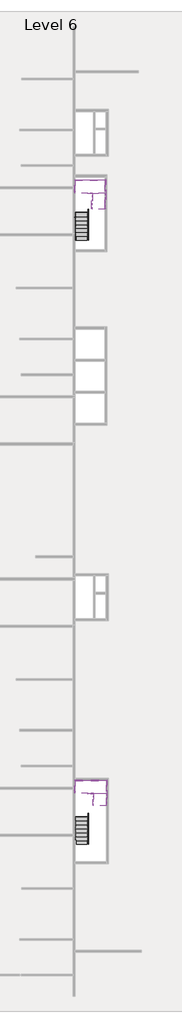
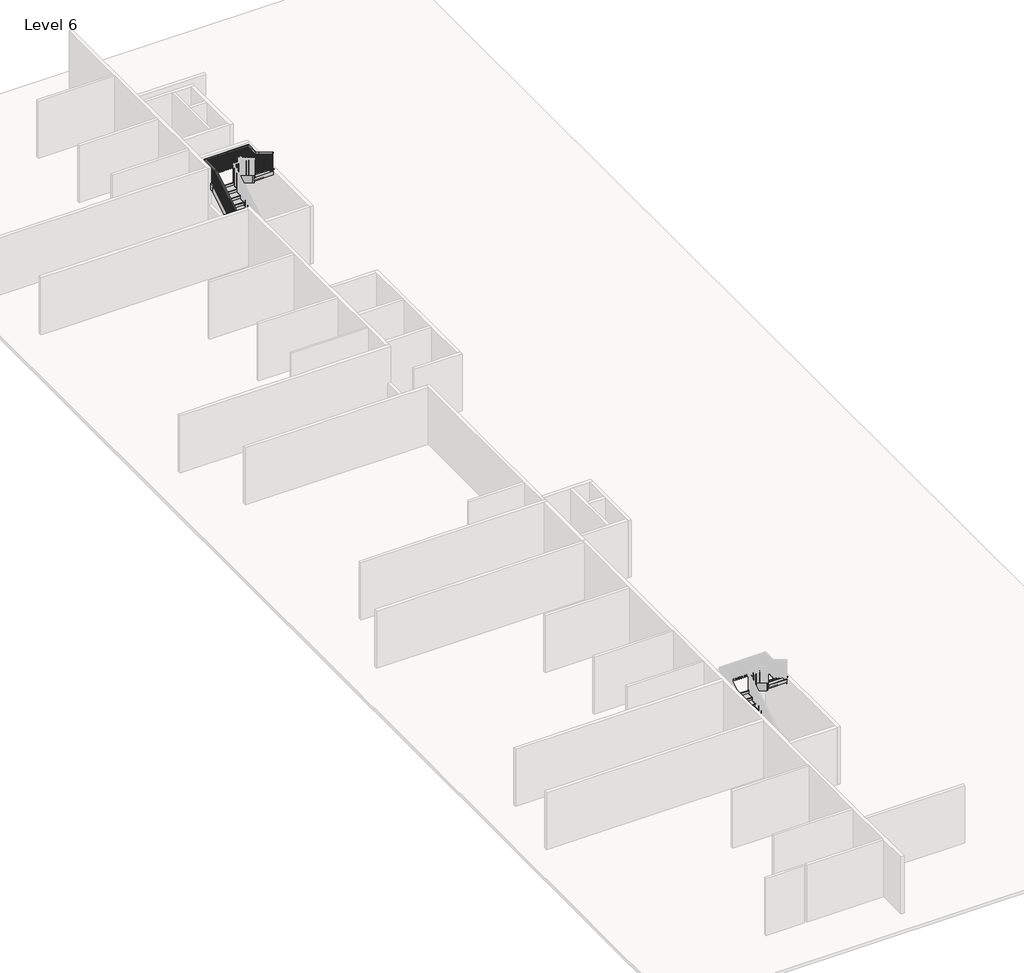
# One storey, part 8 of 8: 16 members, 4 stair flights, 2 slabs, 1 railing.
"""IFC4 building model written with IfcOpenShell, lengths in millimetres."""

from ifc_helpers import new_model, si_unit, frame, origin, place, context, project, spatial, polyline, outline, extrude, faceted_brep, transform, mapped, element, save
from components import non_monolithic_landing_f4425cc3, non_monolithic_landing_d932be8a, stair_flight_a1121a25, stair_flight_592be736, stair_flight_ee9ddb45, stair_flight_fe606327

model = new_model("IFC4")

# Units and contexts
model_context = context("Model", 3, world=origin())
ifc_project = project(units=[si_unit("LENGTHUNIT", "METRE", prefix="MILLI")], contexts=[model_context])

# Site, building, storey
site = spatial("IfcSite", under=ifc_project)
building = spatial("IfcBuilding", under=site)
storey = spatial("IfcBuildingStorey", under=building, Name="Level 6", Elevation=40474.6172466)

# Members
placement = place(None, origin())
element("IfcMember", 1, ObjectType="Stringer - 2\" Width", at=placement, inside=storey, context=model_context, shape_type="SweptSolid", body=[
    extrude(outline(polyline([(-23154.3851539, 40474.6172466), (-23154.3851539, 40686.7317586), (-19467.0440987, 42921.4839133), (-19381.8896422, 42616.6839133), (-22916.2996422, 40474.6172466), (-23154.3851539, 40474.6172466)])), frame((-3668.2415084, 0.0, 0.0), z_axis=(1.0, 0.0, 0.0), x_axis=(0.0, 1.0, 0.0)), (0.0, 0.0, 1.0), 50.8),
])
element("IfcMember", 2, ObjectType="Stringer - 2\" Width", at=placement, inside=storey, context=model_context, shape_type="SweptSolid", body=[
    extrude(outline(polyline([(-23154.3851539, 40474.6172466), (-23154.3851539, 40686.7317586), (-19572.9851539, 42857.2772131), (-19572.9851539, 42500.8684516), (-22916.2996422, 40474.6172466), (-23154.3851539, 40474.6172466)])), frame((-2703.0415084, 0.0, 0.0), z_axis=(1.0, 0.0, 0.0), x_axis=(0.0, 1.0, 0.0)), (0.0, 0.0, 1.0), 50.8),
])
element("IfcMember", 3, ObjectType="Stringer - 2\" Width", at=placement, inside=storey, context=model_context, shape_type="SweptSolid", body=[
    extrude(outline(polyline([(-19297.9262092, 42921.4839133), (-19383.0806657, 42616.6839133), (-20360.3851539, 43208.9896637), (-20360.3851539, 43565.3984252), (-19297.9262092, 42921.4839133)])), frame((-1382.2415084, 0.0, 0.0), z_axis=(1.0, 0.0, 0.0), x_axis=(0.0, 1.0, 0.0)), (0.0, 0.0, 1.0), 50.8),
])
element("IfcMember", 4, ObjectType="Stringer - 2\" Width", at=placement, inside=storey, context=model_context, shape_type="SweptSolid", body=[
    extrude(outline(polyline([(-19522.1851539, 43057.3984252), (-19522.1851539, 42700.9896637), (-20360.3851539, 43208.9896637), (-20360.3851539, 43565.3984252), (-19522.1851539, 43057.3984252)])), frame((-2347.4415084, 0.0, 0.0), z_axis=(1.0, 0.0, 0.0), x_axis=(0.0, 1.0, 0.0)), (0.0, 0.0, 1.0), 50.8),
])
element("IfcMember", 5, ObjectType="Stringer - 2\" Width", at=placement, inside=storey, context=model_context, shape_type="Brep", body=[
    faceted_brep([(-1382.2415084, -19297.9262092, 42921.4839133), (-1331.4415084, -19297.9262092, 42921.4839133), (-1331.4415084, -18556.9851539, 42921.4839133), (-1382.2415084, -18607.7851539, 42921.4839133), (-1382.2415084, -19383.0806657, 42616.6839133), (-1382.2415084, -18607.7851539, 42616.6839133), (-1331.4415084, -19383.0806657, 42616.6839133), (-1331.4415084, -18556.9851539, 42616.6839133)], [[[0, 1, 2, 3]], [[4, 0, 3, 5]], [[6, 4, 5, 7]], [[1, 6, 7, 2]], [[1, 0, 4, 6]], [[2, 7, 5, 3]]]),
])
element("IfcMember", 6, ObjectType="Stringer - 2\" Width", at=placement, inside=storey, context=model_context, shape_type="SweptSolid", body=[
    extrude(outline(polyline([(-1331.4415084, -18556.9851539), (-1382.2415084, -18607.7851539), (-3617.4415084, -18607.7851539), (-3668.2415084, -18556.9851539), (-1331.4415084, -18556.9851539)])), frame((0.0, 0.0, 42616.6839133), z_axis=(0.0, 0.0, 1.0), x_axis=(1.0, 0.0, 0.0)), (0.0, 0.0, 1.0), 304.8),
])
element("IfcMember", 7, ObjectType="Stringer - 2\" Width", at=placement, inside=storey, context=model_context, shape_type="Brep", body=[
    faceted_brep([(-3617.4415084, -18607.7851539, 42921.4839133), (-3668.2415084, -18556.9851539, 42921.4839133), (-3668.2415084, -19467.0440987, 42921.4839133), (-3617.4415084, -19467.0440987, 42921.4839133), (-3617.4415084, -18607.7851539, 42616.6839133), (-3617.4415084, -19381.8896422, 42616.6839133), (-3668.2415084, -18556.9851539, 42616.6839133), (-3668.2415084, -19381.8896422, 42616.6839133)], [[[0, 1, 2, 3]], [[4, 0, 3, 5]], [[6, 4, 5, 7]], [[1, 6, 7, 2]], [[1, 0, 4, 6]], [[2, 7, 5, 3]]]),
])
element("IfcMember", 8, ObjectType="Stringer - 2\" Width", at=placement, inside=storey, context=model_context, shape_type="SweptSolid", body=[
    extrude(outline(polyline([(-2703.0415084, -19572.9851539), (-2703.0415084, -19522.1851539), (-2347.4415084, -19522.1851539), (-2347.4415084, -19572.9851539), (-2703.0415084, -19572.9851539)])), frame((0.0, 0.0, 42616.6839133), z_axis=(0.0, 0.0, 1.0), x_axis=(1.0, 0.0, 0.0)), (0.0, 0.0, 1.0), 304.8),
])
element("IfcMember", 9, ObjectType="Stringer - 2\" Width", at=placement, inside=storey, context=model_context, shape_type="SweptSolid", body=[
    extrude(outline(polyline([(19841.9216096, 40474.6172466), (19841.9216096, 40686.7317586), (23249.8626649, 42752.1505799), (23335.0171214, 42447.3505799), (20080.0071214, 40474.6172466), (19841.9216096, 40474.6172466)])), frame((-3668.2415084, 0.0, 0.0), z_axis=(1.0, 0.0, 0.0), x_axis=(0.0, 1.0, 0.0)), (0.0, 0.0, 1.0), 50.8),
])
element("IfcMember", 10, ObjectType="Stringer - 2\" Width", at=placement, inside=storey, context=model_context, shape_type="SweptSolid", body=[
    extrude(outline(polyline([(19841.9216096, 40474.6172466), (19841.9216096, 40686.7317586), (23143.9216096, 42687.9438798), (23143.9216096, 42331.5351183), (20080.0071214, 40474.6172466), (19841.9216096, 40474.6172466)])), frame((-2703.0415084, 0.0, 0.0), z_axis=(1.0, 0.0, 0.0), x_axis=(0.0, 1.0, 0.0)), (0.0, 0.0, 1.0), 50.8),
])
element("IfcMember", 11, ObjectType="Stringer - 2\" Width", at=placement, inside=storey, context=model_context, shape_type="SweptSolid", body=[
    extrude(outline(polyline([(23418.9805543, 42752.1505799), (23333.8260978, 42447.3505799), (22077.1216096, 43208.9896637), (22077.1216096, 43565.3984252), (23418.9805543, 42752.1505799)])), frame((-1483.8415084, 0.0, 0.0), z_axis=(1.0, 0.0, 0.0), x_axis=(0.0, 1.0, 0.0)), (0.0, 0.0, 1.0), 50.8),
])
element("IfcMember", 12, ObjectType="Stringer - 2\" Width", at=placement, inside=storey, context=model_context, shape_type="SweptSolid", body=[
    extrude(outline(polyline([(23194.7216096, 42888.0650919), (23194.7216096, 42531.6563304), (22077.1216096, 43208.9896637), (22077.1216096, 43565.3984252), (23194.7216096, 42888.0650919)])), frame((-2449.0415084, 0.0, 0.0), z_axis=(1.0, 0.0, 0.0), x_axis=(0.0, 1.0, 0.0)), (0.0, 0.0, 1.0), 50.8),
])
element("IfcMember", 13, ObjectType="Stringer - 2\" Width", at=placement, inside=storey, context=model_context, shape_type="Brep", body=[
    faceted_brep([(-1483.8415084, 23418.9805543, 42752.1505799), (-1433.0415084, 23418.9805543, 42752.1505799), (-1433.0415084, 24159.9216096, 42752.1505799), (-1483.8415084, 24109.1216096, 42752.1505799), (-1483.8415084, 23333.8260978, 42447.3505799), (-1483.8415084, 24109.1216096, 42447.3505799), (-1433.0415084, 23333.8260978, 42447.3505799), (-1433.0415084, 24159.9216096, 42447.3505799)], [[[0, 1, 2, 3]], [[4, 0, 3, 5]], [[6, 4, 5, 7]], [[1, 6, 7, 2]], [[1, 0, 4, 6]], [[2, 7, 5, 3]]]),
])
element("IfcMember", 14, ObjectType="Stringer - 2\" Width", at=placement, inside=storey, context=model_context, shape_type="SweptSolid", body=[
    extrude(outline(polyline([(-1433.0415084, 24159.9216096), (-1483.8415084, 24109.1216096), (-3617.4415084, 24109.1216096), (-3668.2415084, 24159.9216096), (-1433.0415084, 24159.9216096)])), frame((0.0, 0.0, 42447.3505799), z_axis=(0.0, 0.0, 1.0), x_axis=(1.0, 0.0, 0.0)), (0.0, 0.0, 1.0), 304.8),
])
element("IfcMember", 15, ObjectType="Stringer - 2\" Width", at=placement, inside=storey, context=model_context, shape_type="Brep", body=[
    faceted_brep([(-3617.4415084, 24109.1216096, 42752.1505799), (-3668.2415084, 24159.9216096, 42752.1505799), (-3668.2415084, 23249.8626649, 42752.1505799), (-3617.4415084, 23249.8626649, 42752.1505799), (-3617.4415084, 24109.1216096, 42447.3505799), (-3617.4415084, 23335.0171214, 42447.3505799), (-3668.2415084, 24159.9216096, 42447.3505799), (-3668.2415084, 23335.0171214, 42447.3505799)], [[[0, 1, 2, 3]], [[4, 0, 3, 5]], [[6, 4, 5, 7]], [[1, 6, 7, 2]], [[1, 0, 4, 6]], [[2, 7, 5, 3]]]),
])
element("IfcMember", 16, ObjectType="Stringer - 2\" Width", at=placement, inside=storey, context=model_context, shape_type="SweptSolid", body=[
    extrude(outline(polyline([(-2703.0415084, 23143.9216096), (-2703.0415084, 23194.7216096), (-2449.0415084, 23194.7216096), (-2449.0415084, 23143.9216096), (-2703.0415084, 23143.9216096)])), frame((0.0, 0.0, 42447.3505799), z_axis=(0.0, 0.0, 1.0), x_axis=(1.0, 0.0, 0.0)), (0.0, 0.0, 1.0), 304.8),
])

# Railing
element("IfcRailing", 17, ObjectType="Handrail - Rectangular", at=placement, inside=storey, context=model_context, shape_type="SolidModel", body=[
    faceted_brep([(-3617.4415084, 19841.9216096, 41558.3505799), (-3617.4415084, 19841.9216096, 41498.9491197), (-3566.6415084, 19841.9216096, 41498.9491197), (-3566.6415084, 19841.9216096, 41558.3505799), (-3617.4415084, 23194.7216096, 43590.3505799), (-3617.4415084, 23208.914019, 43539.5505799), (-3566.6415084, 23208.914019, 43539.5505799), (-3566.6415084, 23194.7216096, 43590.3505799), (-3617.4415084, 24109.1216096, 43590.3505799), (-3617.4415084, 24109.1216096, 43539.5505799), (-3566.6415084, 24058.3216096, 43539.5505799), (-3566.6415084, 24058.3216096, 43590.3505799), (-1483.8415084, 24109.1216096, 43590.3505799), (-1483.8415084, 24109.1216096, 43539.5505799), (-1534.6415084, 24058.3216096, 43539.5505799), (-1534.6415084, 24058.3216096, 43590.3505799), (-1483.8415084, 23474.1216096, 43590.3505799), (-1483.8415084, 23459.9292002, 43539.5505799), (-1534.6415084, 23459.9292002, 43539.5505799), (-1534.6415084, 23474.1216096, 43590.3505799), (-1483.8415084, 23194.7216096, 43759.6839133), (-1483.8415084, 23168.3918824, 43716.2398634), (-1534.6415084, 23168.3918824, 43716.2398634), (-1534.6415084, 23194.7216096, 43759.6839133), (-1483.8415084, 22077.1216096, 44437.0172466), (-1534.6415084, 22077.1216096, 44437.0172466), (-1534.6415084, 22077.1216096, 44377.6157863), (-1483.8415084, 22077.1216096, 44377.6157863)], [[[0, 1, 2, 3]], [[1, 0, 4, 5]], [[2, 1, 5, 6]], [[3, 2, 6, 7]], [[0, 3, 7, 4]], [[5, 4, 8, 9]], [[6, 5, 9, 10]], [[7, 6, 10, 11]], [[4, 7, 11, 8]], [[9, 8, 12, 13]], [[10, 9, 13, 14]], [[11, 10, 14, 15]], [[8, 11, 15, 12]], [[13, 12, 16, 17]], [[14, 13, 17, 18]], [[15, 14, 18, 19]], [[12, 15, 19, 16]], [[17, 16, 20, 21]], [[18, 17, 21, 22]], [[19, 18, 22, 23]], [[16, 19, 23, 20]], [[24, 25, 26, 27]], [[21, 20, 24, 27]], [[22, 21, 27, 26]], [[23, 22, 26, 25]], [[20, 23, 25, 24]]]),
    extrude(outline(polyline([(22188.2466096, 44310.2673015), (22188.2466096, 43353.2839133), (22169.1966096, 43353.2839133), (22169.1966096, 44321.812756), (22188.2466096, 44310.2673015)])), frame((-1518.7665084, 0.0, 0.0), z_axis=(1.0, 0.0, 0.0), x_axis=(0.0, 1.0, 0.0)), (0.0, 0.0, 1.0), 19.05),
    extrude(outline(polyline([(22289.8466096, 44248.6915439), (22289.8466096, 43353.2839133), (22270.7966096, 43353.2839133), (22270.7966096, 44260.2369985), (22289.8466096, 44248.6915439)])), frame((-1518.7665084, 0.0, 0.0), z_axis=(1.0, 0.0, 0.0), x_axis=(0.0, 1.0, 0.0)), (0.0, 0.0, 1.0), 19.05),
    extrude(outline(polyline([(22391.4466096, 44187.1157863), (22391.4466096, 43183.9505799), (22372.3966096, 43183.9505799), (22372.3966096, 44198.6612409), (22391.4466096, 44187.1157863)])), frame((-1518.7665084, 0.0, 0.0), z_axis=(1.0, 0.0, 0.0), x_axis=(0.0, 1.0, 0.0)), (0.0, 0.0, 1.0), 19.05),
    extrude(outline(polyline([(22493.0466096, 44125.5400288), (22493.0466096, 43183.9505799), (22473.9966096, 43183.9505799), (22473.9966096, 44137.0854833), (22493.0466096, 44125.5400288)])), frame((-1518.7665084, 0.0, 0.0), z_axis=(1.0, 0.0, 0.0), x_axis=(0.0, 1.0, 0.0)), (0.0, 0.0, 1.0), 19.05),
    extrude(outline(polyline([(22594.6466096, 44063.9642712), (22594.6466096, 43183.9505799), (22575.5966096, 43183.9505799), (22575.5966096, 44075.5097257), (22594.6466096, 44063.9642712)])), frame((-1518.7665084, 0.0, 0.0), z_axis=(1.0, 0.0, 0.0), x_axis=(0.0, 1.0, 0.0)), (0.0, 0.0, 1.0), 19.05),
    extrude(outline(polyline([(22696.2466096, 44002.3885136), (22696.2466096, 43014.6172466), (22677.1966096, 43014.6172466), (22677.1966096, 44013.9339682), (22696.2466096, 44002.3885136)])), frame((-1518.7665084, 0.0, 0.0), z_axis=(1.0, 0.0, 0.0), x_axis=(0.0, 1.0, 0.0)), (0.0, 0.0, 1.0), 19.05),
    extrude(outline(polyline([(22797.8466096, 43940.812756), (22797.8466096, 43014.6172466), (22778.7966096, 43014.6172466), (22778.7966096, 43952.3582106), (22797.8466096, 43940.812756)])), frame((-1518.7665084, 0.0, 0.0), z_axis=(1.0, 0.0, 0.0), x_axis=(0.0, 1.0, 0.0)), (0.0, 0.0, 1.0), 19.05),
    extrude(outline(polyline([(22899.4466096, 43879.2369985), (22899.4466096, 43014.6172466), (22880.3966096, 43014.6172466), (22880.3966096, 43890.782453), (22899.4466096, 43879.2369985)])), frame((-1518.7665084, 0.0, 0.0), z_axis=(1.0, 0.0, 0.0), x_axis=(0.0, 1.0, 0.0)), (0.0, 0.0, 1.0), 19.05),
    extrude(outline(polyline([(23001.0466096, 43817.6612409), (23001.0466096, 42845.2839133), (22981.9966096, 42845.2839133), (22981.9966096, 43829.2066954), (23001.0466096, 43817.6612409)])), frame((-1518.7665084, 0.0, 0.0), z_axis=(1.0, 0.0, 0.0), x_axis=(0.0, 1.0, 0.0)), (0.0, 0.0, 1.0), 19.05),
    extrude(outline(polyline([(23102.6466096, 43756.0854833), (23102.6466096, 42845.2839133), (23083.5966096, 42845.2839133), (23083.5966096, 43767.6309379), (23102.6466096, 43756.0854833)])), frame((-1518.7665084, 0.0, 0.0), z_axis=(1.0, 0.0, 0.0), x_axis=(0.0, 1.0, 0.0)), (0.0, 0.0, 1.0), 19.05),
    extrude(outline(polyline([(23280.4466096, 43648.3279076), (23280.4466096, 42675.9505799), (23261.3966096, 42675.9505799), (23261.3966096, 43659.8733621), (23280.4466096, 43648.3279076)])), frame((-1518.7665084, 0.0, 0.0), z_axis=(1.0, 0.0, 0.0), x_axis=(0.0, 1.0, 0.0)), (0.0, 0.0, 1.0), 19.05),
    extrude(outline(polyline([(23382.0466096, 43586.75215), (23382.0466096, 42675.9505799), (23362.9966096, 42675.9505799), (23362.9966096, 43598.2976045), (23382.0466096, 43586.75215)])), frame((-1518.7665084, 0.0, 0.0), z_axis=(1.0, 0.0, 0.0), x_axis=(0.0, 1.0, 0.0)), (0.0, 0.0, 1.0), 19.05),
    extrude(outline(polyline([(-1499.7165084, 23483.6466096), (-1499.7165084, 23464.5966096), (-1518.7665084, 23464.5966096), (-1518.7665084, 23483.6466096), (-1499.7165084, 23483.6466096)])), frame((0.0, 0.0, 42675.9505799), z_axis=(0.0, 0.0, 1.0), x_axis=(1.0, 0.0, 0.0)), (0.0, 0.0, 1.0), 863.6),
    extrude(outline(polyline([(-1499.7165084, 23585.2466096), (-1499.7165084, 23566.1966096), (-1518.7665084, 23566.1966096), (-1518.7665084, 23585.2466096), (-1499.7165084, 23585.2466096)])), frame((0.0, 0.0, 42675.9505799), z_axis=(0.0, 0.0, 1.0), x_axis=(1.0, 0.0, 0.0)), (0.0, 0.0, 1.0), 863.6),
    extrude(outline(polyline([(-1499.7165084, 23686.8466096), (-1499.7165084, 23667.7966096), (-1518.7665084, 23667.7966096), (-1518.7665084, 23686.8466096), (-1499.7165084, 23686.8466096)])), frame((0.0, 0.0, 42675.9505799), z_axis=(0.0, 0.0, 1.0), x_axis=(1.0, 0.0, 0.0)), (0.0, 0.0, 1.0), 863.6),
    extrude(outline(polyline([(-1499.7165084, 23788.4466096), (-1499.7165084, 23769.3966096), (-1518.7665084, 23769.3966096), (-1518.7665084, 23788.4466096), (-1499.7165084, 23788.4466096)])), frame((0.0, 0.0, 42675.9505799), z_axis=(0.0, 0.0, 1.0), x_axis=(1.0, 0.0, 0.0)), (0.0, 0.0, 1.0), 863.6),
    extrude(outline(polyline([(-1499.7165084, 23890.0466096), (-1499.7165084, 23870.9966096), (-1518.7665084, 23870.9966096), (-1518.7665084, 23890.0466096), (-1499.7165084, 23890.0466096)])), frame((0.0, 0.0, 42675.9505799), z_axis=(0.0, 0.0, 1.0), x_axis=(1.0, 0.0, 0.0)), (0.0, 0.0, 1.0), 863.6),
    extrude(outline(polyline([(-1499.7165084, 23991.6466096), (-1499.7165084, 23972.5966096), (-1518.7665084, 23972.5966096), (-1518.7665084, 23991.6466096), (-1499.7165084, 23991.6466096)])), frame((0.0, 0.0, 42675.9505799), z_axis=(0.0, 0.0, 1.0), x_axis=(1.0, 0.0, 0.0)), (0.0, 0.0, 1.0), 863.6),
    extrude(outline(polyline([(-1569.5665084, 24093.2466096), (-1550.5165084, 24093.2466096), (-1550.5165084, 24074.1966096), (-1569.5665084, 24074.1966096), (-1569.5665084, 24093.2466096)])), frame((0.0, 0.0, 42675.9505799), z_axis=(0.0, 0.0, 1.0), x_axis=(1.0, 0.0, 0.0)), (0.0, 0.0, 1.0), 863.6),
    extrude(outline(polyline([(-1671.1665084, 24093.2466096), (-1652.1165084, 24093.2466096), (-1652.1165084, 24074.1966096), (-1671.1665084, 24074.1966096), (-1671.1665084, 24093.2466096)])), frame((0.0, 0.0, 42675.9505799), z_axis=(0.0, 0.0, 1.0), x_axis=(1.0, 0.0, 0.0)), (0.0, 0.0, 1.0), 863.6),
    extrude(outline(polyline([(-1772.7665084, 24093.2466096), (-1753.7165084, 24093.2466096), (-1753.7165084, 24074.1966096), (-1772.7665084, 24074.1966096), (-1772.7665084, 24093.2466096)])), frame((0.0, 0.0, 42675.9505799), z_axis=(0.0, 0.0, 1.0), x_axis=(1.0, 0.0, 0.0)), (0.0, 0.0, 1.0), 863.6),
    extrude(outline(polyline([(-1874.3665084, 24093.2466096), (-1855.3165084, 24093.2466096), (-1855.3165084, 24074.1966096), (-1874.3665084, 24074.1966096), (-1874.3665084, 24093.2466096)])), frame((0.0, 0.0, 42675.9505799), z_axis=(0.0, 0.0, 1.0), x_axis=(1.0, 0.0, 0.0)), (0.0, 0.0, 1.0), 863.6),
    extrude(outline(polyline([(-1975.9665084, 24093.2466096), (-1956.9165084, 24093.2466096), (-1956.9165084, 24074.1966096), (-1975.9665084, 24074.1966096), (-1975.9665084, 24093.2466096)])), frame((0.0, 0.0, 42675.9505799), z_axis=(0.0, 0.0, 1.0), x_axis=(1.0, 0.0, 0.0)), (0.0, 0.0, 1.0), 863.6),
    extrude(outline(polyline([(-2077.5665084, 24093.2466096), (-2058.5165084, 24093.2466096), (-2058.5165084, 24074.1966096), (-2077.5665084, 24074.1966096), (-2077.5665084, 24093.2466096)])), frame((0.0, 0.0, 42675.9505799), z_axis=(0.0, 0.0, 1.0), x_axis=(1.0, 0.0, 0.0)), (0.0, 0.0, 1.0), 863.6),
    extrude(outline(polyline([(-2179.1665084, 24093.2466096), (-2160.1165084, 24093.2466096), (-2160.1165084, 24074.1966096), (-2179.1665084, 24074.1966096), (-2179.1665084, 24093.2466096)])), frame((0.0, 0.0, 42675.9505799), z_axis=(0.0, 0.0, 1.0), x_axis=(1.0, 0.0, 0.0)), (0.0, 0.0, 1.0), 863.6),
    extrude(outline(polyline([(-2280.7665084, 24093.2466096), (-2261.7165084, 24093.2466096), (-2261.7165084, 24074.1966096), (-2280.7665084, 24074.1966096), (-2280.7665084, 24093.2466096)])), frame((0.0, 0.0, 42675.9505799), z_axis=(0.0, 0.0, 1.0), x_axis=(1.0, 0.0, 0.0)), (0.0, 0.0, 1.0), 863.6),
    extrude(outline(polyline([(-2382.3665084, 24093.2466096), (-2363.3165084, 24093.2466096), (-2363.3165084, 24074.1966096), (-2382.3665084, 24074.1966096), (-2382.3665084, 24093.2466096)])), frame((0.0, 0.0, 42675.9505799), z_axis=(0.0, 0.0, 1.0), x_axis=(1.0, 0.0, 0.0)), (0.0, 0.0, 1.0), 863.6),
    extrude(outline(polyline([(-2483.9665084, 24093.2466096), (-2464.9165084, 24093.2466096), (-2464.9165084, 24074.1966096), (-2483.9665084, 24074.1966096), (-2483.9665084, 24093.2466096)])), frame((0.0, 0.0, 42675.9505799), z_axis=(0.0, 0.0, 1.0), x_axis=(1.0, 0.0, 0.0)), (0.0, 0.0, 1.0), 863.6),
    extrude(outline(polyline([(-2585.5665084, 24093.2466096), (-2566.5165084, 24093.2466096), (-2566.5165084, 24074.1966096), (-2585.5665084, 24074.1966096), (-2585.5665084, 24093.2466096)])), frame((0.0, 0.0, 42675.9505799), z_axis=(0.0, 0.0, 1.0), x_axis=(1.0, 0.0, 0.0)), (0.0, 0.0, 1.0), 863.6),
    extrude(outline(polyline([(-2687.1665084, 24093.2466096), (-2668.1165084, 24093.2466096), (-2668.1165084, 24074.1966096), (-2687.1665084, 24074.1966096), (-2687.1665084, 24093.2466096)])), frame((0.0, 0.0, 42675.9505799), z_axis=(0.0, 0.0, 1.0), x_axis=(1.0, 0.0, 0.0)), (0.0, 0.0, 1.0), 863.6),
    extrude(outline(polyline([(-2788.7665084, 24093.2466096), (-2769.7165084, 24093.2466096), (-2769.7165084, 24074.1966096), (-2788.7665084, 24074.1966096), (-2788.7665084, 24093.2466096)])), frame((0.0, 0.0, 42675.9505799), z_axis=(0.0, 0.0, 1.0), x_axis=(1.0, 0.0, 0.0)), (0.0, 0.0, 1.0), 863.6),
    extrude(outline(polyline([(-2890.3665084, 24093.2466096), (-2871.3165084, 24093.2466096), (-2871.3165084, 24074.1966096), (-2890.3665084, 24074.1966096), (-2890.3665084, 24093.2466096)])), frame((0.0, 0.0, 42675.9505799), z_axis=(0.0, 0.0, 1.0), x_axis=(1.0, 0.0, 0.0)), (0.0, 0.0, 1.0), 863.6),
    extrude(outline(polyline([(-2991.9665084, 24093.2466096), (-2972.9165084, 24093.2466096), (-2972.9165084, 24074.1966096), (-2991.9665084, 24074.1966096), (-2991.9665084, 24093.2466096)])), frame((0.0, 0.0, 42675.9505799), z_axis=(0.0, 0.0, 1.0), x_axis=(1.0, 0.0, 0.0)), (0.0, 0.0, 1.0), 863.6),
    extrude(outline(polyline([(-3093.5665084, 24093.2466096), (-3074.5165084, 24093.2466096), (-3074.5165084, 24074.1966096), (-3093.5665084, 24074.1966096), (-3093.5665084, 24093.2466096)])), frame((0.0, 0.0, 42675.9505799), z_axis=(0.0, 0.0, 1.0), x_axis=(1.0, 0.0, 0.0)), (0.0, 0.0, 1.0), 863.6),
    extrude(outline(polyline([(-3195.1665084, 24093.2466096), (-3176.1165084, 24093.2466096), (-3176.1165084, 24074.1966096), (-3195.1665084, 24074.1966096), (-3195.1665084, 24093.2466096)])), frame((0.0, 0.0, 42675.9505799), z_axis=(0.0, 0.0, 1.0), x_axis=(1.0, 0.0, 0.0)), (0.0, 0.0, 1.0), 863.6),
    extrude(outline(polyline([(-3296.7665084, 24093.2466096), (-3277.7165084, 24093.2466096), (-3277.7165084, 24074.1966096), (-3296.7665084, 24074.1966096), (-3296.7665084, 24093.2466096)])), frame((0.0, 0.0, 42675.9505799), z_axis=(0.0, 0.0, 1.0), x_axis=(1.0, 0.0, 0.0)), (0.0, 0.0, 1.0), 863.6),
    extrude(outline(polyline([(-3398.3665084, 24093.2466096), (-3379.3165084, 24093.2466096), (-3379.3165084, 24074.1966096), (-3398.3665084, 24074.1966096), (-3398.3665084, 24093.2466096)])), frame((0.0, 0.0, 42675.9505799), z_axis=(0.0, 0.0, 1.0), x_axis=(1.0, 0.0, 0.0)), (0.0, 0.0, 1.0), 863.6),
    extrude(outline(polyline([(-3499.9665084, 24093.2466096), (-3480.9165084, 24093.2466096), (-3480.9165084, 24074.1966096), (-3499.9665084, 24074.1966096), (-3499.9665084, 24093.2466096)])), frame((0.0, 0.0, 42675.9505799), z_axis=(0.0, 0.0, 1.0), x_axis=(1.0, 0.0, 0.0)), (0.0, 0.0, 1.0), 863.6),
    extrude(outline(polyline([(-3601.5665084, 23997.9966096), (-3601.5665084, 24017.0466096), (-3582.5165084, 24017.0466096), (-3582.5165084, 23997.9966096), (-3601.5665084, 23997.9966096)])), frame((0.0, 0.0, 42675.9505799), z_axis=(0.0, 0.0, 1.0), x_axis=(1.0, 0.0, 0.0)), (0.0, 0.0, 1.0), 863.6),
    extrude(outline(polyline([(-3601.5665084, 23896.3966096), (-3601.5665084, 23915.4466096), (-3582.5165084, 23915.4466096), (-3582.5165084, 23896.3966096), (-3601.5665084, 23896.3966096)])), frame((0.0, 0.0, 42675.9505799), z_axis=(0.0, 0.0, 1.0), x_axis=(1.0, 0.0, 0.0)), (0.0, 0.0, 1.0), 863.6),
    extrude(outline(polyline([(-3601.5665084, 23794.7966096), (-3601.5665084, 23813.8466096), (-3582.5165084, 23813.8466096), (-3582.5165084, 23794.7966096), (-3601.5665084, 23794.7966096)])), frame((0.0, 0.0, 42675.9505799), z_axis=(0.0, 0.0, 1.0), x_axis=(1.0, 0.0, 0.0)), (0.0, 0.0, 1.0), 863.6),
    extrude(outline(polyline([(-3601.5665084, 23693.1966096), (-3601.5665084, 23712.2466096), (-3582.5165084, 23712.2466096), (-3582.5165084, 23693.1966096), (-3601.5665084, 23693.1966096)])), frame((0.0, 0.0, 42675.9505799), z_axis=(0.0, 0.0, 1.0), x_axis=(1.0, 0.0, 0.0)), (0.0, 0.0, 1.0), 863.6),
    extrude(outline(polyline([(-3601.5665084, 23591.5966096), (-3601.5665084, 23610.6466096), (-3582.5165084, 23610.6466096), (-3582.5165084, 23591.5966096), (-3601.5665084, 23591.5966096)])), frame((0.0, 0.0, 42675.9505799), z_axis=(0.0, 0.0, 1.0), x_axis=(1.0, 0.0, 0.0)), (0.0, 0.0, 1.0), 863.6),
    extrude(outline(polyline([(-3601.5665084, 23489.9966096), (-3601.5665084, 23509.0466096), (-3582.5165084, 23509.0466096), (-3582.5165084, 23489.9966096), (-3601.5665084, 23489.9966096)])), frame((0.0, 0.0, 42675.9505799), z_axis=(0.0, 0.0, 1.0), x_axis=(1.0, 0.0, 0.0)), (0.0, 0.0, 1.0), 863.6),
    extrude(outline(polyline([(-3601.5665084, 23388.3966096), (-3601.5665084, 23407.4466096), (-3582.5165084, 23407.4466096), (-3582.5165084, 23388.3966096), (-3601.5665084, 23388.3966096)])), frame((0.0, 0.0, 42675.9505799), z_axis=(0.0, 0.0, 1.0), x_axis=(1.0, 0.0, 0.0)), (0.0, 0.0, 1.0), 863.6),
    extrude(outline(polyline([(-3601.5665084, 23286.7966096), (-3601.5665084, 23305.8466096), (-3582.5165084, 23305.8466096), (-3582.5165084, 23286.7966096), (-3601.5665084, 23286.7966096)])), frame((0.0, 0.0, 42675.9505799), z_axis=(0.0, 0.0, 1.0), x_axis=(1.0, 0.0, 0.0)), (0.0, 0.0, 1.0), 863.6),
    extrude(outline(polyline([(23102.6466096, 43475.1460894), (23102.6466096, 42506.6172466), (23083.5966096, 42506.6172466), (23083.5966096, 43463.6006348), (23102.6466096, 43475.1460894)])), frame((-3601.5665084, 0.0, 0.0), z_axis=(1.0, 0.0, 0.0), x_axis=(0.0, 1.0, 0.0)), (0.0, 0.0, 1.0), 19.05),
    extrude(outline(polyline([(23001.0466096, 43413.5703318), (23001.0466096, 42506.6172466), (22981.9966096, 42506.6172466), (22981.9966096, 43402.0248773), (23001.0466096, 43413.5703318)])), frame((-3601.5665084, 0.0, 0.0), z_axis=(1.0, 0.0, 0.0), x_axis=(0.0, 1.0, 0.0)), (0.0, 0.0, 1.0), 19.05),
    extrude(outline(polyline([(22899.4466096, 43351.9945742), (22899.4466096, 42337.2839133), (22880.3966096, 42337.2839133), (22880.3966096, 43340.4491197), (22899.4466096, 43351.9945742)])), frame((-3601.5665084, 0.0, 0.0), z_axis=(1.0, 0.0, 0.0), x_axis=(0.0, 1.0, 0.0)), (0.0, 0.0, 1.0), 19.05),
    extrude(outline(polyline([(22797.8466096, 43290.4188166), (22797.8466096, 42337.2839133), (22778.7966096, 42337.2839133), (22778.7966096, 43278.8733621), (22797.8466096, 43290.4188166)])), frame((-3601.5665084, 0.0, 0.0), z_axis=(1.0, 0.0, 0.0), x_axis=(0.0, 1.0, 0.0)), (0.0, 0.0, 1.0), 19.05),
    extrude(outline(polyline([(22696.2466096, 43228.8430591), (22696.2466096, 42337.2839133), (22677.1966096, 42337.2839133), (22677.1966096, 43217.2976045), (22696.2466096, 43228.8430591)])), frame((-3601.5665084, 0.0, 0.0), z_axis=(1.0, 0.0, 0.0), x_axis=(0.0, 1.0, 0.0)), (0.0, 0.0, 1.0), 19.05),
    extrude(outline(polyline([(22594.6466096, 43167.2673015), (22594.6466096, 42167.9505799), (22575.5966096, 42167.9505799), (22575.5966096, 43155.721847), (22594.6466096, 43167.2673015)])), frame((-3601.5665084, 0.0, 0.0), z_axis=(1.0, 0.0, 0.0), x_axis=(0.0, 1.0, 0.0)), (0.0, 0.0, 1.0), 19.05),
    extrude(outline(polyline([(22493.0466096, 43105.6915439), (22493.0466096, 42167.9505799), (22473.9966096, 42167.9505799), (22473.9966096, 43094.1460894), (22493.0466096, 43105.6915439)])), frame((-3601.5665084, 0.0, 0.0), z_axis=(1.0, 0.0, 0.0), x_axis=(0.0, 1.0, 0.0)), (0.0, 0.0, 1.0), 19.05),
    extrude(outline(polyline([(22391.4466096, 43044.1157863), (22391.4466096, 42167.9505799), (22372.3966096, 42167.9505799), (22372.3966096, 43032.5703318), (22391.4466096, 43044.1157863)])), frame((-3601.5665084, 0.0, 0.0), z_axis=(1.0, 0.0, 0.0), x_axis=(0.0, 1.0, 0.0)), (0.0, 0.0, 1.0), 19.05),
    extrude(outline(polyline([(22289.8466096, 42982.5400288), (22289.8466096, 41998.6172466), (22270.7966096, 41998.6172466), (22270.7966096, 42970.9945742), (22289.8466096, 42982.5400288)])), frame((-3601.5665084, 0.0, 0.0), z_axis=(1.0, 0.0, 0.0), x_axis=(0.0, 1.0, 0.0)), (0.0, 0.0, 1.0), 19.05),
    extrude(outline(polyline([(22188.2466096, 42920.9642712), (22188.2466096, 41998.6172466), (22169.1966096, 41998.6172466), (22169.1966096, 42909.4188166), (22188.2466096, 42920.9642712)])), frame((-3601.5665084, 0.0, 0.0), z_axis=(1.0, 0.0, 0.0), x_axis=(0.0, 1.0, 0.0)), (0.0, 0.0, 1.0), 19.05),
    extrude(outline(polyline([(22086.6466096, 42859.3885136), (22086.6466096, 41998.6172466), (22067.5966096, 41998.6172466), (22067.5966096, 42847.8430591), (22086.6466096, 42859.3885136)])), frame((-3601.5665084, 0.0, 0.0), z_axis=(1.0, 0.0, 0.0), x_axis=(0.0, 1.0, 0.0)), (0.0, 0.0, 1.0), 19.05),
    extrude(outline(polyline([(21985.0466096, 42797.812756), (21985.0466096, 41829.2839133), (21965.9966096, 41829.2839133), (21965.9966096, 42786.2673015), (21985.0466096, 42797.812756)])), frame((-3601.5665084, 0.0, 0.0), z_axis=(1.0, 0.0, 0.0), x_axis=(0.0, 1.0, 0.0)), (0.0, 0.0, 1.0), 19.05),
    extrude(outline(polyline([(21883.4466096, 42736.2369985), (21883.4466096, 41829.2839133), (21864.3966096, 41829.2839133), (21864.3966096, 42724.6915439), (21883.4466096, 42736.2369985)])), frame((-3601.5665084, 0.0, 0.0), z_axis=(1.0, 0.0, 0.0), x_axis=(0.0, 1.0, 0.0)), (0.0, 0.0, 1.0), 19.05),
    extrude(outline(polyline([(21781.8466096, 42674.6612409), (21781.8466096, 41659.9505799), (21762.7966096, 41659.9505799), (21762.7966096, 42663.1157863), (21781.8466096, 42674.6612409)])), frame((-3601.5665084, 0.0, 0.0), z_axis=(1.0, 0.0, 0.0), x_axis=(0.0, 1.0, 0.0)), (0.0, 0.0, 1.0), 19.05),
    extrude(outline(polyline([(21680.2466096, 42613.0854833), (21680.2466096, 41659.9505799), (21661.1966096, 41659.9505799), (21661.1966096, 42601.5400288), (21680.2466096, 42613.0854833)])), frame((-3601.5665084, 0.0, 0.0), z_axis=(1.0, 0.0, 0.0), x_axis=(0.0, 1.0, 0.0)), (0.0, 0.0, 1.0), 19.05),
    extrude(outline(polyline([(21578.6466096, 42551.5097257), (21578.6466096, 41659.9505799), (21559.5966096, 41659.9505799), (21559.5966096, 42539.9642712), (21578.6466096, 42551.5097257)])), frame((-3601.5665084, 0.0, 0.0), z_axis=(1.0, 0.0, 0.0), x_axis=(0.0, 1.0, 0.0)), (0.0, 0.0, 1.0), 19.05),
    extrude(outline(polyline([(21477.0466096, 42489.9339682), (21477.0466096, 41490.6172466), (21457.9966096, 41490.6172466), (21457.9966096, 42478.3885136), (21477.0466096, 42489.9339682)])), frame((-3601.5665084, 0.0, 0.0), z_axis=(1.0, 0.0, 0.0), x_axis=(0.0, 1.0, 0.0)), (0.0, 0.0, 1.0), 19.05),
    extrude(outline(polyline([(21375.4466096, 42428.3582106), (21375.4466096, 41490.6172466), (21356.3966096, 41490.6172466), (21356.3966096, 42416.812756), (21375.4466096, 42428.3582106)])), frame((-3601.5665084, 0.0, 0.0), z_axis=(1.0, 0.0, 0.0), x_axis=(0.0, 1.0, 0.0)), (0.0, 0.0, 1.0), 19.05),
    extrude(outline(polyline([(21273.8466096, 42366.782453), (21273.8466096, 41490.6172466), (21254.7966096, 41490.6172466), (21254.7966096, 42355.2369985), (21273.8466096, 42366.782453)])), frame((-3601.5665084, 0.0, 0.0), z_axis=(1.0, 0.0, 0.0), x_axis=(0.0, 1.0, 0.0)), (0.0, 0.0, 1.0), 19.05),
    extrude(outline(polyline([(21172.2466096, 42305.2066954), (21172.2466096, 41321.2839133), (21153.1966096, 41321.2839133), (21153.1966096, 42293.6612409), (21172.2466096, 42305.2066954)])), frame((-3601.5665084, 0.0, 0.0), z_axis=(1.0, 0.0, 0.0), x_axis=(0.0, 1.0, 0.0)), (0.0, 0.0, 1.0), 19.05),
    extrude(outline(polyline([(21070.6466096, 42243.6309379), (21070.6466096, 41321.2839133), (21051.5966096, 41321.2839133), (21051.5966096, 42232.0854833), (21070.6466096, 42243.6309379)])), frame((-3601.5665084, 0.0, 0.0), z_axis=(1.0, 0.0, 0.0), x_axis=(0.0, 1.0, 0.0)), (0.0, 0.0, 1.0), 19.05),
    extrude(outline(polyline([(20969.0466096, 42182.0551803), (20969.0466096, 41321.2839133), (20949.9966096, 41321.2839133), (20949.9966096, 42170.5097257), (20969.0466096, 42182.0551803)])), frame((-3601.5665084, 0.0, 0.0), z_axis=(1.0, 0.0, 0.0), x_axis=(0.0, 1.0, 0.0)), (0.0, 0.0, 1.0), 19.05),
    extrude(outline(polyline([(20867.4466096, 42120.4794227), (20867.4466096, 41151.9505799), (20848.3966096, 41151.9505799), (20848.3966096, 42108.9339682), (20867.4466096, 42120.4794227)])), frame((-3601.5665084, 0.0, 0.0), z_axis=(1.0, 0.0, 0.0), x_axis=(0.0, 1.0, 0.0)), (0.0, 0.0, 1.0), 19.05),
    extrude(outline(polyline([(20765.8466096, 42058.9036651), (20765.8466096, 41151.9505799), (20746.7966096, 41151.9505799), (20746.7966096, 42047.3582106), (20765.8466096, 42058.9036651)])), frame((-3601.5665084, 0.0, 0.0), z_axis=(1.0, 0.0, 0.0), x_axis=(0.0, 1.0, 0.0)), (0.0, 0.0, 1.0), 19.05),
    extrude(outline(polyline([(20664.2466096, 41997.3279076), (20664.2466096, 40982.6172466), (20645.1966096, 40982.6172466), (20645.1966096, 41985.782453), (20664.2466096, 41997.3279076)])), frame((-3601.5665084, 0.0, 0.0), z_axis=(1.0, 0.0, 0.0), x_axis=(0.0, 1.0, 0.0)), (0.0, 0.0, 1.0), 19.05),
    extrude(outline(polyline([(20562.6466096, 41935.75215), (20562.6466096, 40982.6172466), (20543.5966096, 40982.6172466), (20543.5966096, 41924.2066954), (20562.6466096, 41935.75215)])), frame((-3601.5665084, 0.0, 0.0), z_axis=(1.0, 0.0, 0.0), x_axis=(0.0, 1.0, 0.0)), (0.0, 0.0, 1.0), 19.05),
    extrude(outline(polyline([(20461.0466096, 41874.1763924), (20461.0466096, 40982.6172466), (20441.9966096, 40982.6172466), (20441.9966096, 41862.6309379), (20461.0466096, 41874.1763924)])), frame((-3601.5665084, 0.0, 0.0), z_axis=(1.0, 0.0, 0.0), x_axis=(0.0, 1.0, 0.0)), (0.0, 0.0, 1.0), 19.05),
    extrude(outline(polyline([(20359.4466096, 41812.6006348), (20359.4466096, 40813.2839133), (20340.3966096, 40813.2839133), (20340.3966096, 41801.0551803), (20359.4466096, 41812.6006348)])), frame((-3601.5665084, 0.0, 0.0), z_axis=(1.0, 0.0, 0.0), x_axis=(0.0, 1.0, 0.0)), (0.0, 0.0, 1.0), 19.05),
    extrude(outline(polyline([(20257.8466096, 41751.0248773), (20257.8466096, 40813.2839133), (20238.7966096, 40813.2839133), (20238.7966096, 41739.4794227), (20257.8466096, 41751.0248773)])), frame((-3601.5665084, 0.0, 0.0), z_axis=(1.0, 0.0, 0.0), x_axis=(0.0, 1.0, 0.0)), (0.0, 0.0, 1.0), 19.05),
    extrude(outline(polyline([(20156.2466096, 41689.4491197), (20156.2466096, 40813.2839133), (20137.1966096, 40813.2839133), (20137.1966096, 41677.9036651), (20156.2466096, 41689.4491197)])), frame((-3601.5665084, 0.0, 0.0), z_axis=(1.0, 0.0, 0.0), x_axis=(0.0, 1.0, 0.0)), (0.0, 0.0, 1.0), 19.05),
    extrude(outline(polyline([(20054.6466096, 41627.8733621), (20054.6466096, 40643.9505799), (20035.5966096, 40643.9505799), (20035.5966096, 41616.3279076), (20054.6466096, 41627.8733621)])), frame((-3601.5665084, 0.0, 0.0), z_axis=(1.0, 0.0, 0.0), x_axis=(0.0, 1.0, 0.0)), (0.0, 0.0, 1.0), 19.05),
    extrude(outline(polyline([(19953.0466096, 41566.2976045), (19953.0466096, 40643.9505799), (19933.9966096, 40643.9505799), (19933.9966096, 41554.75215), (19953.0466096, 41566.2976045)])), frame((-3601.5665084, 0.0, 0.0), z_axis=(1.0, 0.0, 0.0), x_axis=(0.0, 1.0, 0.0)), (0.0, 0.0, 1.0), 19.05),
    extrude(outline(polyline([(23204.2466096, 43694.5097257), (23204.2466096, 42675.9505799), (23185.1966096, 42675.9505799), (23185.1966096, 43706.0551803), (23204.2466096, 43694.5097257)])), frame((-1518.7665084, 0.0, 0.0), z_axis=(1.0, 0.0, 0.0), x_axis=(0.0, 1.0, 0.0)), (0.0, 0.0, 1.0), 19.05),
    extrude(outline(polyline([(-1518.7665084, 24093.2466096), (-1499.7165084, 24093.2466096), (-1499.7165084, 24074.1966096), (-1518.7665084, 24074.1966096), (-1518.7665084, 24093.2466096)])), frame((0.0, 0.0, 42675.9505799), z_axis=(0.0, 0.0, 1.0), x_axis=(1.0, 0.0, 0.0)), (0.0, 0.0, 1.0), 863.6),
    extrude(outline(polyline([(-3601.5665084, 24074.1966096), (-3601.5665084, 24093.2466096), (-3582.5165084, 24093.2466096), (-3582.5165084, 24074.1966096), (-3601.5665084, 24074.1966096)])), frame((0.0, 0.0, 42675.9505799), z_axis=(0.0, 0.0, 1.0), x_axis=(1.0, 0.0, 0.0)), (0.0, 0.0, 1.0), 863.6),
    extrude(outline(polyline([(23204.2466096, 43536.721847), (23204.2466096, 42675.9505799), (23185.1966096, 42675.9505799), (23185.1966096, 43525.1763924), (23204.2466096, 43536.721847)])), frame((-3601.5665084, 0.0, 0.0), z_axis=(1.0, 0.0, 0.0), x_axis=(0.0, 1.0, 0.0)), (0.0, 0.0, 1.0), 19.05),
    extrude(outline(polyline([(22096.1716096, 44366.0703318), (22096.1716096, 43353.2839133), (22077.1216096, 43353.2839133), (22077.1216096, 44377.6157863), (22096.1716096, 44366.0703318)])), frame((-1518.7665084, 0.0, 0.0), z_axis=(1.0, 0.0, 0.0), x_axis=(0.0, 1.0, 0.0)), (0.0, 0.0, 1.0), 19.05),
    extrude(outline(polyline([(19860.9716096, 41510.4945742), (19860.9716096, 40643.9505799), (19841.9216096, 40643.9505799), (19841.9216096, 41498.9491197), (19860.9716096, 41510.4945742)])), frame((-3601.5665084, 0.0, 0.0), z_axis=(1.0, 0.0, 0.0), x_axis=(0.0, 1.0, 0.0)), (0.0, 0.0, 1.0), 19.05),
])

# Slabs
non_monolithic_landing_shape = non_monolithic_landing_f4425cc3(model_context)
element("IfcSlab", 18, ObjectType="Non-Monolithic Landing", at=placement, inside=storey, context=model_context, shape_type="MappedRepresentation", body=[
    mapped(non_monolithic_landing_shape, transform((0.0, 0.0, 0.0), x_axis=(1.0, 0.0, 0.0), y_axis=(0.0, 1.0, 0.0), z_axis=(0.0, 0.0, 1.0))),
])
non_monolithic_landing_2_shape = non_monolithic_landing_d932be8a(model_context)
element("IfcSlab", 19, ObjectType="Non-Monolithic Landing", at=placement, inside=storey, context=model_context, shape_type="MappedRepresentation", body=[
    mapped(non_monolithic_landing_2_shape, transform((0.0, 0.0, 0.0), x_axis=(1.0, 0.0, 0.0), y_axis=(0.0, 1.0, 0.0), z_axis=(0.0, 0.0, 1.0))),
])

# Stair flights
stair_flight_shape = stair_flight_a1121a25(model_context)
element("IfcStairFlight", 20, ObjectType="2\" Tread 1\" Nosing 1/4\" Riser", at=placement, inside=storey, context=model_context, shape_type="MappedRepresentation", body=[
    mapped(stair_flight_shape, transform((0.0, 0.0, 0.0), x_axis=(1.0, 0.0, 0.0), y_axis=(0.0, 1.0, 0.0), z_axis=(0.0, 0.0, 1.0))),
])
stair_flight_2_shape = stair_flight_592be736(model_context)
element("IfcStairFlight", 21, ObjectType="2\" Tread 1\" Nosing 1/4\" Riser", at=placement, inside=storey, context=model_context, shape_type="MappedRepresentation", body=[
    mapped(stair_flight_2_shape, transform((0.0, 0.0, 0.0), x_axis=(1.0, 0.0, 0.0), y_axis=(0.0, 1.0, 0.0), z_axis=(0.0, 0.0, 1.0))),
])
stair_flight_3_shape = stair_flight_ee9ddb45(model_context)
element("IfcStairFlight", 22, ObjectType="2\" Tread 1\" Nosing 1/4\" Riser", at=placement, inside=storey, context=model_context, shape_type="MappedRepresentation", body=[
    mapped(stair_flight_3_shape, transform((0.0, 0.0, 0.0), x_axis=(1.0, 0.0, 0.0), y_axis=(0.0, 1.0, 0.0), z_axis=(0.0, 0.0, 1.0))),
])
stair_flight_4_shape = stair_flight_fe606327(model_context)
element("IfcStairFlight", 23, ObjectType="2\" Tread 1\" Nosing 1/4\" Riser", at=placement, inside=storey, context=model_context, shape_type="MappedRepresentation", body=[
    mapped(stair_flight_4_shape, transform((0.0, 0.0, 0.0), x_axis=(1.0, 0.0, 0.0), y_axis=(0.0, 1.0, 0.0), z_axis=(0.0, 0.0, 1.0))),
])

save(model, "model.ifc")

# Revit data of these elements
# Type "Handrail - Rectangular"
#   Assembly Code = "C2010400"
#   built-in parameter 1008612 = 0.0416667 (stored number, unit not read)
#   built-in parameter 1008611 = 0.0416667 (stored number, unit not read)
#   built-in parameter 1008609 = 0.333333 (stored number, unit not read)
#   built-in parameter 1008604 = 0.166667 (stored number, unit not read)
#   built-in parameter 1008603 = 0.166667 (stored number, unit not read)
#   Railing Height = 3' - 0"
#   built-in parameter 1008630 = 2
#   built-in parameter 1008610 = 2
#   built-in parameter 1008618 = Baluster - Square : 3/4"
# Elements 1, 2, 3, 4, 5, 6, 7, 8, 9, 10, 11, 12, 13, 14, 15, 16 (IfcMember, "Stringer - 2\" Width")
#   Phase Created = New Construction
# Element 17 (IfcRailing, "Handrail - Rectangular")
#   Phase Created = New Construction
# Elements 18, 19 (IfcSlab, "Non-Monolithic Landing")
#   Phase Created = New Construction
# Elements 20, 21, 22, 23 (IfcStairFlight, "2\" Tread 1\" Nosing 1/4\" Riser")
#   Phase Created = New Construction
